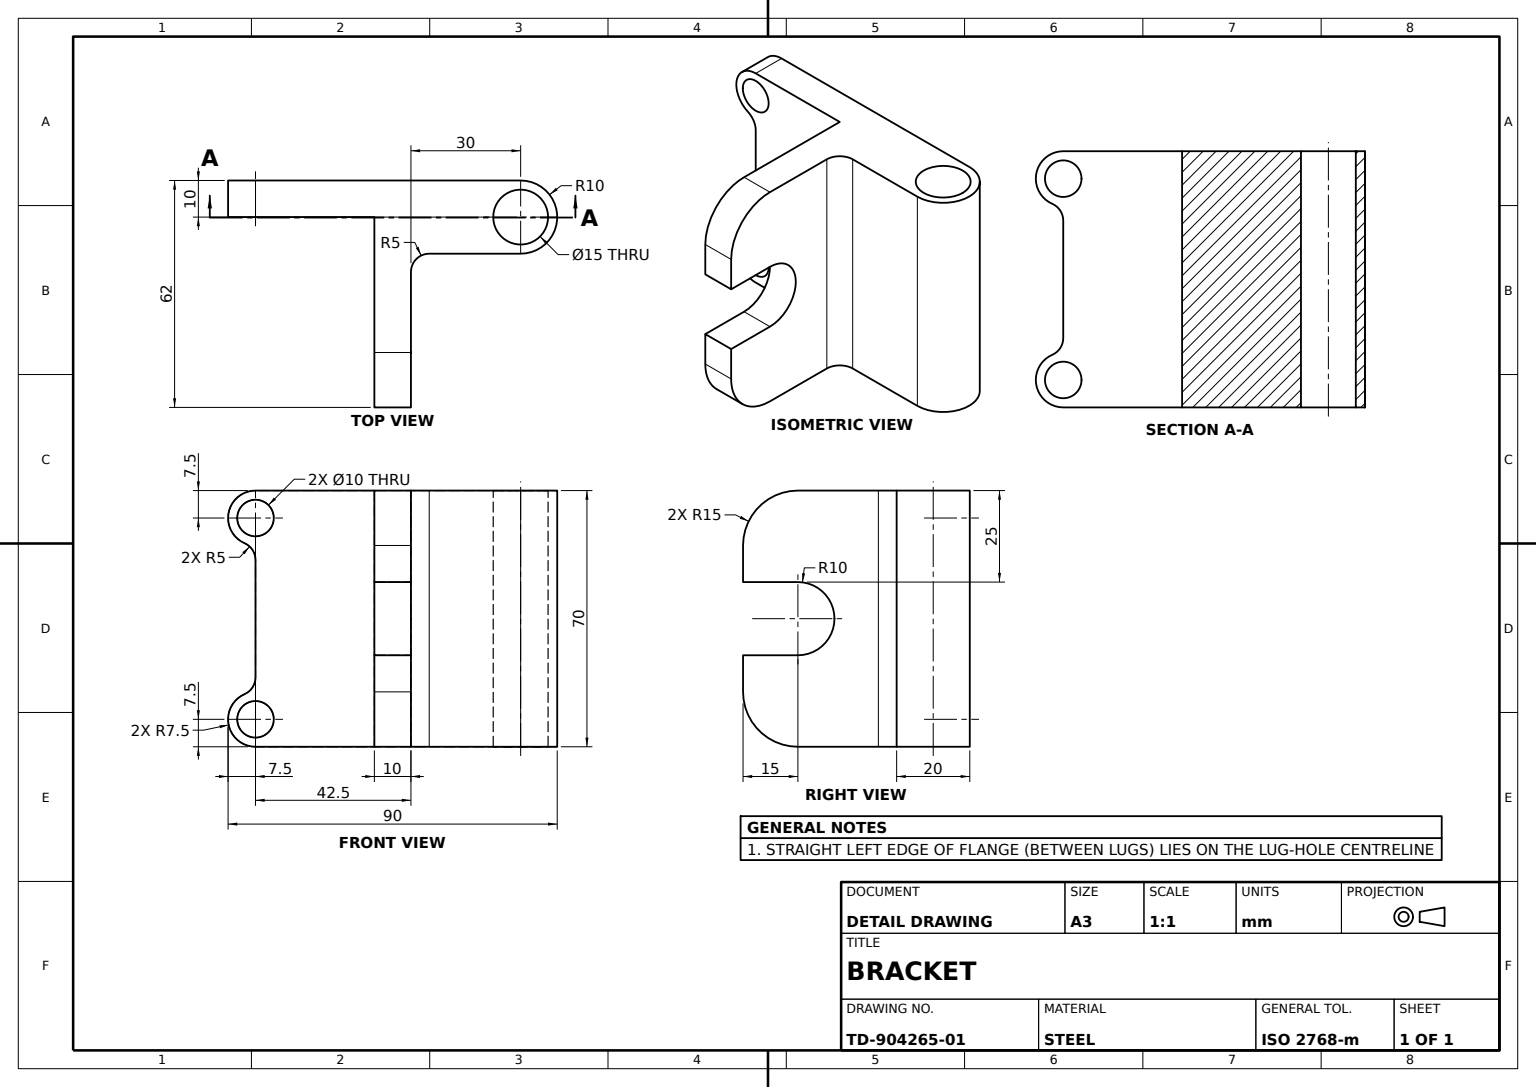
SolidWorks part; units mm, degrees
material "Plain Carbon Steel"
ref_plane "Front Plane" through (0, 0, 0) normal (0, 0, 1) x (1, 0, 0)
ref_plane "Top Plane" through (0, 0, 0) normal (0, 1, 0) x (1, 0, 0)
ref_plane "Right Plane" through (0, 0, 0) normal (1, 0, 0) x (0, 0, -1)
sketch "Base Plate Sketch" plane through (0, 0, 0) normal (0, 0, 1) x (1, 0, 0)
  line L0 (0, 0) -> (47, 0)
  line L1 (62, 15) -> (62, 25)
  line L2 (47, 70) -> (0, 70)
  line L3 (0, 70) -> (0, 0)
  line L5 (62, 45) -> (47, 45)
  line L6 (62, 45) -> (62, 55)
  line L7 (47, 25) -> (62, 25)
  arc A0 (62, 15) -> (47, 0) centre (47, 15) cw
  arc A1 (62, 55) -> (47, 70) centre (47, 55) ccw
  arc A3 (47, 45) -> (47, 25) centre (47, 35) ccw
  dimension "D1" = 15
  dimension "D2" = 20
  dimension "D3" = 62
extrude "Base Plate" add sketch "Base Plate Sketch" along normal blind 10
sketch "Mounting Flange Sketch" plane through (0, 0, 0) normal (-1, 0, 0) x (0, 0, 1)
  line L0 (10, 70) -> (42.5, 70)
  line L1 (42.5, 70) -> (42.5, 0)
  line L2 (42.5, 0) -> (10, 0)
  line L3 (10, 0) -> (10, 70)
  line L4 (0, 70) -> (0, 0) construction
  dimension "D1" = 42.5
extrude "Mounting Flange" add sketch "Mounting Flange Sketch" against normal blind 10
sketch "Flange Lug Sketch" plane through (10, 0, 0) normal (1, 0, 0) x (0, 0, -1)
  line L0 (-42.5, 35) -> (-42.5, 51.0436)
  line L1 (-42.5, 0) -> (-42.5, 70) construction
  line L2 (-42.5, 35) -> (-42.5, 18.9564)
  line L3 (-42.5, 70) -> (-42.5, 0)
  arc A0 (-42.5, 70) -> (-45.5, 55.6261) centre (-42.5, 62.5) ccw
  arc A1 (-45.5, 14.3739) -> (-42.5, 0) centre (-42.5, 7.5) ccw
  arc A2 (-45.5, 14.3739) -> (-42.5, 18.9564) centre (-47.5, 18.9564) ccw
  arc A3 (-42.5, 51.0436) -> (-45.5, 55.6261) centre (-47.5, 51.0436) ccw
  line M3 (-42.5, 70) -> (-42.5, 0)
  dimension "D1" = 5
  dimension "D2" = 7.5
extrude "Flange Lugs" add sketch "Flange Lug Sketch" against normal blind 10 contours A3 A0 M3 | A2 A1 M3
sketch "Mounting Hole Sketch" plane through (10, 0, 0) normal (1, 0, 0) x (0, 0, -1)
  circle A0 centre (-42.5, 62.5) radius 5
  circle A1 centre (-42.5, 7.5) radius 5
  dimension "D1" = 10
extrude "Mounting Holes" cut sketch "Mounting Hole Sketch" against normal blind 10
sketch "Upright Web Sketch" plane through (0, 0, 0) normal (-1, 0, 0) x (0, 0, 1)
  line L0 (0, 70) -> (-30, 70)
  line L1 (-30, 70) -> (-30, 0)
  line L2 (-30, 0) -> (0, 0)
  line L3 (0, 0) -> (0, 70)
  line L4 (0, 70) -> (0, 0) construction
  dimension "D1" = 30
extrude "Upright Web" add sketch "Upright Web Sketch" against normal blind 25
sketch "Web Relief Cut Sketch" plane through (0, 70, 0) normal (0, 1, 0) x (1, 0, 0)
  line L0 (25, 30) -> (20, 30)
  line L1 (25, 30) -> (0, 30) construction
  line L2 (20, 30) -> (20, 0)
  line L3 (20, 0) -> (25, 0)
  line L4 (25, 0) -> (25, 30)
  line L5 (0, -42.5) -> (0, 30) construction
  dimension "D1" = 20
extrude "Web Relief Cut" cut sketch "Web Relief Cut Sketch" against normal blind 70
sketch "Rounded Arm Sketch" plane through (0, 70, 0) normal (0, 1, 0) x (1, 0, 0)
  line L0 (20, 0) -> (25, 0)
  line L1 (47, 0) -> (20, 0) construction
  line L3 (20, 0) -> (20, 5)
  line L4 (20, 30) -> (20, 0) construction
  arc A0 (20, 5) -> (25, 0) centre (25, 5) ccw
  dimension "D1" = 5
extrude "Rounded Arm" add sketch "Rounded Arm Sketch" against normal blind 70
sketch "Bore Boss Sketch" plane through (0, 70, 0) normal (0, 1, 0) x (1, 0, 0)
  line L0 (20, 30) -> (0, 30) construction
  line L1 (0, 30) -> (20, 30)
  arc A0 (20, 30) -> (0, 30) centre (10, 30) ccw
extrude "Bore Boss" add sketch "Bore Boss Sketch" against normal blind 70
sketch "Bore Sketch" plane through (0, 70, 0) normal (0, 1, 0) x (1, 0, 0)
  circle A0 centre (10, 30) radius 7.5
  dimension "D1" = 15
extrude "Through Bore" cut sketch "Bore Sketch" against normal blind 70
